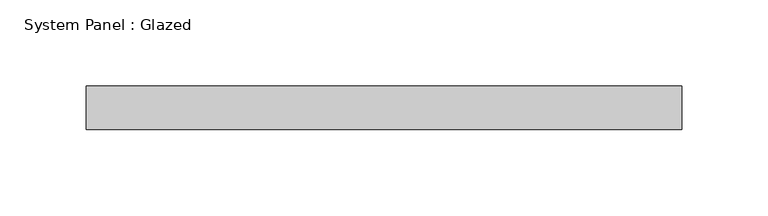
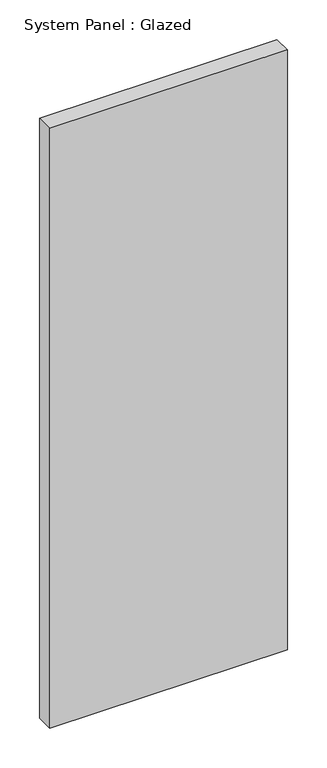
"""IFC4 building model written with IfcOpenShell, lengths in millimetres: plate geometry, System Panel : Glazed."""

from ifc_helpers import new_model, si_unit, origin, origin_with_axes, place, context, project, spatial, polyline, outline, extrude, source, transform, mapped, element, save


def system_panel_glazed_404bb2e9(model_context):
    return source(origin(), model_context, "Body", "SweptSolid", [
        extrude(outline(polyline([(173.0712159, 19.05), (-173.0712159, 19.05), (-173.0712159, 44.45), (173.0712159, 44.45), (173.0712159, 19.05)])), origin_with_axes(), (0.0, 0.0, 1.0), 923.1640555),
    ])


if __name__ == "__main__":
    model = new_model("IFC4")
    model_context = context("Model", 3, world=origin())
    ifc_project = project(units=[si_unit("LENGTHUNIT", "METRE", prefix="MILLI")], contexts=[model_context])
    site = spatial("IfcSite", under=ifc_project)
    building = spatial("IfcBuilding", under=site)
    placement = place(None, origin())
    system_panel_glazed_shape = system_panel_glazed_404bb2e9(model_context)
    element("IfcPlate", 1, ObjectType="System Panel : Glazed", at=placement, inside=building, context=model_context, shape_type="MappedRepresentation", body=[
        mapped(system_panel_glazed_shape, transform((0.0, 0.0, 0.0), x_axis=(1.0, 0.0, 0.0), y_axis=(0.0, 1.0, 0.0), z_axis=(0.0, 0.0, 1.0))),
    ])
    save(model, "model.ifc")

# Revit data of these elements
# Type "System Panel : Glazed"
#   Construction Type Id = "GSP4R"
#   Analytic Construction = "1/8 in Pilkington single glazing"
#   Visual Light Transmittance = 0.9
#   Solar Heat Gain Coefficient = 0.86
#   Heat Transfer Coefficient (U) = 1.18115 BTU/(h·ft²·°F)
# Element 1 (IfcPlate, "System Panel : Glazed")
#   Materials on its faces: "Glass"
# Materials
#   "Glass": class "Glass", colour RGB 0 128 192, transparency 0.75, Description = "Soda Lime Glass", Cost = 0
